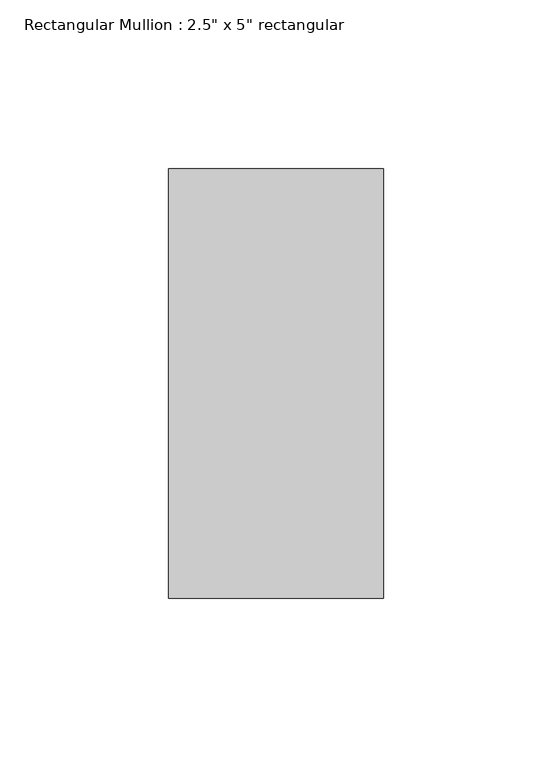
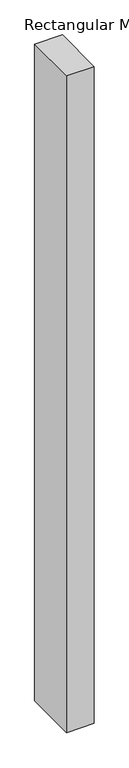
"""IFC4 building model written with IfcOpenShell, lengths in millimetres: member geometry."""

from ifc_helpers import new_model, si_unit, frame, origin, place, context, project, spatial, polyline, outline, extrude, source, transform, mapped, element, save


def member_75b26f99(model_context):
    return source(origin(), model_context, "Body", "SweptSolid", [
        extrude(outline(polyline([(0.0, 63.5), (0.0, -63.5), (-63.5, -63.5), (-63.5, 63.5), (0.0, 63.5)])), frame((0.0, 0.0, -1599.2829369), z_axis=(0.0, 0.0, 1.0), x_axis=(1.0, 0.0, 0.0)), (0.0, 0.0, 1.0), 1599.2829369),
    ])


if __name__ == "__main__":
    model = new_model("IFC4")
    model_context = context("Model", 3, world=origin())
    ifc_project = project(units=[si_unit("LENGTHUNIT", "METRE", prefix="MILLI")], contexts=[model_context])
    site = spatial("IfcSite", under=ifc_project)
    building = spatial("IfcBuilding", under=site)
    placement = place(None, origin())
    member_shape = member_75b26f99(model_context)
    element("IfcMember", 1, ObjectType="Rectangular Mullion : 2.5\" x 5\" rectangular", at=placement, inside=building, context=model_context, shape_type="MappedRepresentation", body=[
        mapped(member_shape, transform((0.0, 0.0, 0.0), x_axis=(1.0, 0.0, 0.0), y_axis=(0.0, 1.0, 0.0), z_axis=(0.0, 0.0, 1.0))),
    ])
    save(model, "model.ifc")

# Revit data of these elements
# Type "Rectangular Mullion : 2.5\" x 5\" rectangular"
#   built-in parameter 1007304 = 0.416667 (stored number, unit not read)
#   built-in parameter 1007301 = 0.104167 (stored number, unit not read)
#   built-in parameter 1007300 = 0.104167 (stored number, unit not read)
# Element 1 (IfcMember, "Rectangular Mullion : 2.5\" x 5\" rectangular")
#   Materials on its faces: "Aluminum"
# Materials
#   "Aluminum": class "Metal", colour RGB 247 247 247, transparency 0, Description = "Aluminum 6061", Cost = 0
